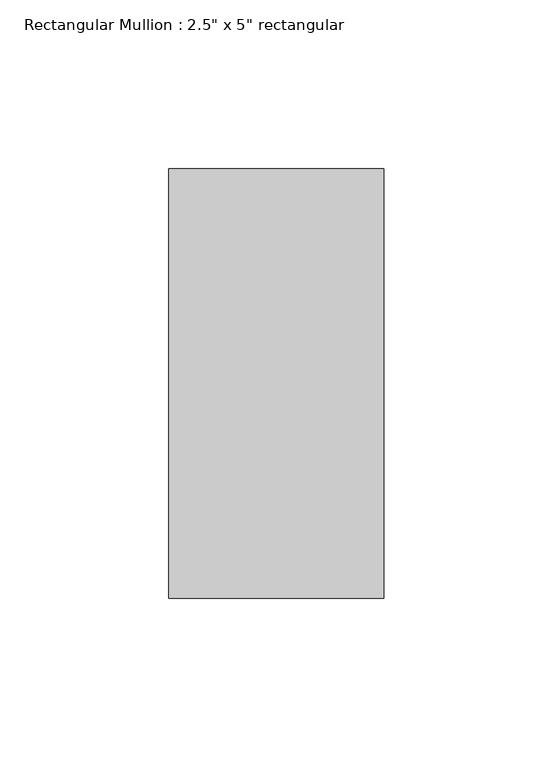
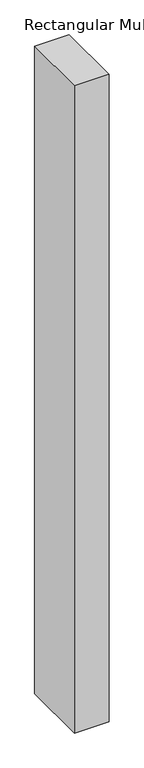
"""IFC4 building model written with IfcOpenShell, lengths in millimetres: member geometry."""

from ifc_helpers import new_model, si_unit, frame, origin, place, context, project, spatial, polyline, outline, extrude, source, transform, mapped, element, save


def member_a6f19fa4(model_context):
    return source(origin(), model_context, "Body", "SweptSolid", [
        extrude(outline(polyline([(0.0, 63.5), (0.0, -63.5), (-63.5, -63.5), (-63.5, 63.5), (0.0, 63.5)])), frame((0.0, 0.0, -1259.4166667), z_axis=(0.0, 0.0, 1.0), x_axis=(1.0, 0.0, 0.0)), (0.0, 0.0, 1.0), 1259.4166667),
    ])


if __name__ == "__main__":
    model = new_model("IFC4")
    model_context = context("Model", 3, world=origin())
    ifc_project = project(units=[si_unit("LENGTHUNIT", "METRE", prefix="MILLI")], contexts=[model_context])
    site = spatial("IfcSite", under=ifc_project)
    building = spatial("IfcBuilding", under=site)
    placement = place(None, origin())
    member_shape = member_a6f19fa4(model_context)
    element("IfcMember", 1, ObjectType="Rectangular Mullion : 2.5\" x 5\" rectangular", at=placement, inside=building, context=model_context, shape_type="MappedRepresentation", body=[
        mapped(member_shape, transform((0.0, 0.0, 0.0), x_axis=(1.0, 0.0, 0.0), y_axis=(0.0, 1.0, 0.0), z_axis=(0.0, 0.0, 1.0))),
    ])
    save(model, "model.ifc")

# Revit data of these elements
# Type "Rectangular Mullion : 2.5\" x 5\" rectangular"
#   built-in parameter 1007304 = 0.416667 (stored number, unit not read)
#   built-in parameter 1007301 = 0.104167 (stored number, unit not read)
#   built-in parameter 1007300 = 0.104167 (stored number, unit not read)
# Element 1 (IfcMember, "Rectangular Mullion : 2.5\" x 5\" rectangular")
#   Materials on its faces: "Aluminum"
# Materials
#   "Aluminum": class "Metal", colour RGB 247 247 247, transparency 0, Description = "Aluminum 6061", Cost = 0
